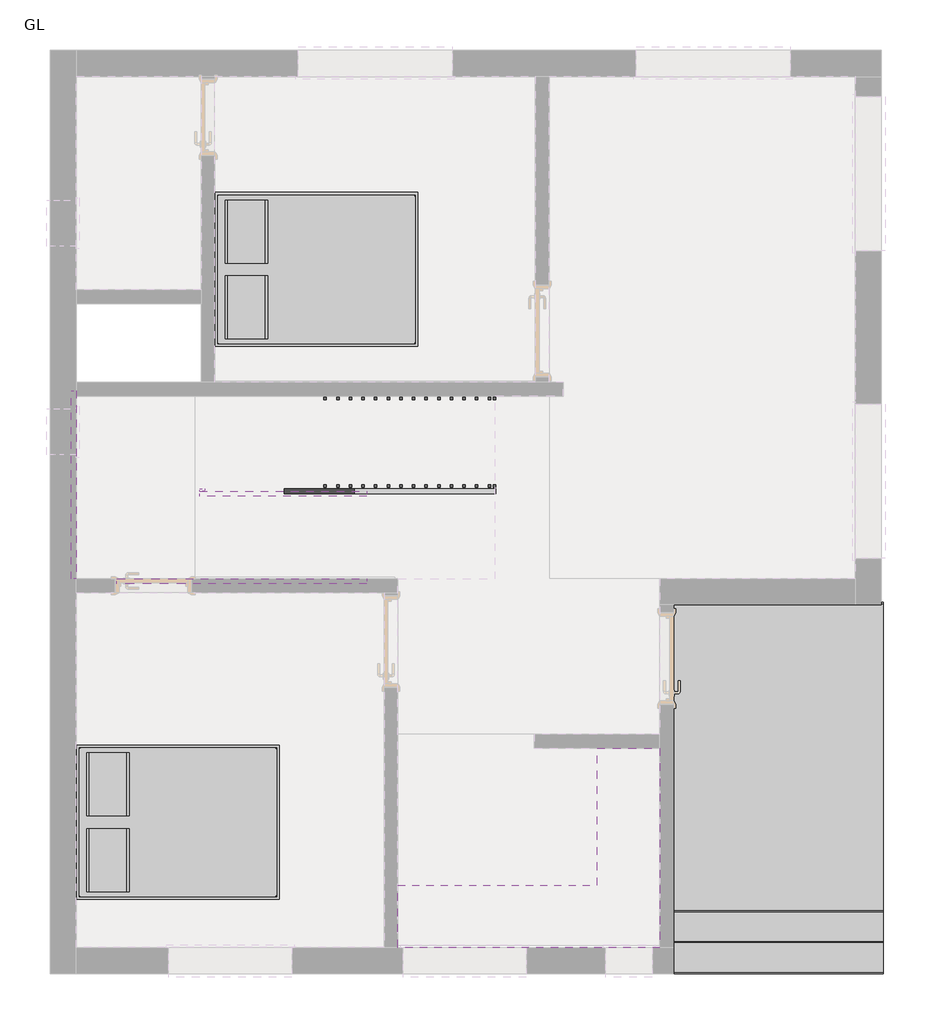
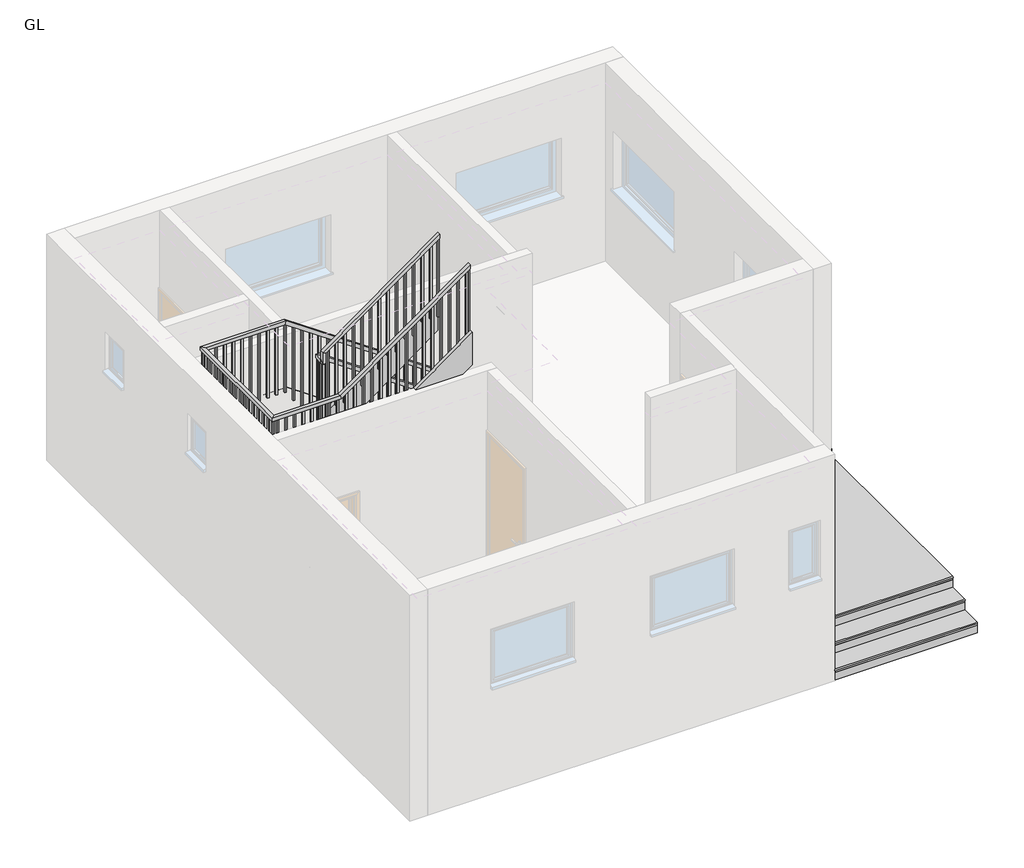
# One storey, part 2 of 2: 6 members, 2 furniture elements, 2 railings, 1 proxy, 1 stair flight.
"""IFC4 building model written with IfcOpenShell, lengths in millimetres."""

from ifc_helpers import new_model, si_unit, frame, origin, place, context, project, spatial, polyline, outline, extrude, faceted_brep, transform, mapped, element, save
from components import generic_models_1_generic_models_1_a00969f3, furniture_bed_1_1525x2007x355mm_queen_b7403446, wood_steps_w_50mm_tread_10mm_nosing_13mm_riser_5aef8f96

model = new_model("IFC4")

# Units and contexts
model_context = context("Model", 3, world=origin())
ifc_project = project(units=[si_unit("LENGTHUNIT", "METRE", prefix="MILLI")], contexts=[model_context])

# Site, building, storey
site = spatial("IfcSite", under=ifc_project)
building = spatial("IfcBuilding", under=site)
storey = spatial("IfcBuildingStorey", under=building, Name="GL", Elevation=0.0)

# Proxy
placement = place(None, origin())
generic_models_1_generic_models_1_shape = generic_models_1_generic_models_1_a00969f3(model_context)
element("IfcBuildingElementProxy", 1, Name="Generic Models 1 : Generic Models 1", ObjectType="Generic Models 1 : Generic Models 1", at=placement, inside=storey, context=model_context, shape_type="MappedRepresentation", body=[
    mapped(generic_models_1_generic_models_1_shape, transform((0.0, 0.0, 0.0), x_axis=(1.0, 0.0, 0.0), y_axis=(0.0, 1.0, 0.0), z_axis=(0.0, 0.0, 1.0))),
])

# Furniture
furniture_bed_1_1525x2007x355mm_queen_shape = furniture_bed_1_1525x2007x355mm_queen_b7403446(model_context)
element("IfcFurniture", 2, ObjectType="Furniture_Bed_1 : 1525x2007x355mm-Queen", at=placement, inside=storey, context=model_context, shape_type="MappedRepresentation", body=[
    mapped(furniture_bed_1_1525x2007x355mm_queen_shape, transform((-8898.6799313, 8340.8671174, 149.9616), x_axis=(0.0, 1.0, 0.0), y_axis=(-1.0, 0.0, 0.0), z_axis=(0.0, 0.0, 1.0))),
])
element("IfcFurniture", 3, ObjectType="Furniture_Bed_1 : 1525x2007x355mm-Queen", at=placement, inside=storey, context=model_context, shape_type="MappedRepresentation", body=[
    mapped(furniture_bed_1_1525x2007x355mm_queen_shape, transform((-10270.2799313, 2866.1131635, 149.9616), x_axis=(0.0, 1.0, 0.0), y_axis=(-1.0, 0.0, 0.0), z_axis=(0.0, 0.0, 1.0))),
])

# Members
element("IfcMember", 4, ObjectType="Stringer-50mm_Width", at=placement, inside=storey, context=model_context, shape_type="SweptSolid", body=[
    extrude(outline(polyline([(0.0, -6888.9904231), (228.9871217, -6888.9904231), (2233.7240638, -9767.6104231), (1746.2809583, -9767.6104231), (0.0, -7260.1097198), (0.0, -6888.9904231)])), frame((0.0, 6457.7656226, 0.0), z_axis=(0.0, 1.0, 0.0), x_axis=(0.0, 0.0, 1.0)), (0.0, 0.0, 1.0), 50.0),
])
element("IfcMember", 5, ObjectType="Stringer-50mm_Width", at=placement, inside=storey, context=model_context, shape_type="SweptSolid", body=[
    extrude(outline(polyline([(-9817.6104231, 6507.7656226), (-9767.6104231, 6507.7656226), (-9767.6104231, 6481.5656226), (-9817.6104231, 6481.5656226), (-9817.6104231, 6507.7656226)])), frame((0.0, 0.0, 1843.7698415), z_axis=(0.0, 0.0, 1.0), x_axis=(1.0, 0.0, 0.0)), (0.0, 0.0, 1.0), 400.0),
])
element("IfcMember", 6, ObjectType="Stringer-50mm_Width", at=placement, inside=storey, context=model_context, shape_type="SweptSolid", body=[
    extrude(outline(polyline([(2441.6210321, -9817.6104231), (1947.0221045, -9817.6104231), (3150.0584681, -8163.4354231), (3644.6573957, -8163.4354231), (2441.6210321, -9817.6104231)])), frame((0.0, 6431.5656226, 0.0), z_axis=(0.0, 1.0, 0.0), x_axis=(0.0, 0.0, 1.0)), (0.0, 0.0, 1.0), 50.0),
])
element("IfcMember", 7, ObjectType="Stringer-50mm_Width", at=placement, inside=storey, context=model_context, shape_type="SweptSolid", body=[
    extrude(outline(polyline([(0.0, -6888.9904231), (228.9871217, -6888.9904231), (2243.7698415, -9782.0352466), (2243.7698415, -10481.9592331), (0.0, -7260.1097198), (0.0, -6888.9904231)])), frame((0.0, 7426.4671174, 0.0), z_axis=(0.0, 1.0, 0.0), x_axis=(0.0, 0.0, 1.0)), (0.0, 0.0, 1.0), 50.0),
])
element("IfcMember", 8, ObjectType="Stringer-50mm_Width", at=placement, inside=storey, context=model_context, shape_type="SweptSolid", body=[
    extrude(outline(polyline([(-11089.3504231, 7476.4671174), (-11039.3504231, 7476.4671174), (-11039.3504231, 5614.7791611), (-11089.3504231, 5614.7791611), (-11089.3504231, 7476.4671174)])), frame((0.0, 0.0, 1843.7698415), z_axis=(0.0, 0.0, 1.0), x_axis=(1.0, 0.0, 0.0)), (0.0, 0.0, 1.0), 400.0),
])
element("IfcMember", 9, ObjectType="Stringer-50mm_Width", at=placement, inside=storey, context=model_context, shape_type="SweptSolid", body=[
    extrude(outline(polyline([(1843.7698415, -9959.5822848), (3150.0584681, -8163.4354231), (3644.6573957, -8163.4354231), (1843.7698415, -10639.6558102), (1843.7698415, -9959.5822848)])), frame((0.0, 5564.7791611, 0.0), z_axis=(0.0, 1.0, 0.0), x_axis=(0.0, 0.0, 1.0)), (0.0, 0.0, 1.0), 50.0),
])

# Railings
element("IfcRailing", 10, ObjectType="1100mm", at=placement, inside=storey, context=model_context, shape_type="SolidModel", body=[
    faceted_brep([(-6888.9904231, 7376.0671174, 1269.3333333), (-6888.9904231, 7376.0671174, 1208.4765973), (-6888.9904231, 7426.0671174, 1208.4765973), (-6888.9904231, 7426.0671174, 1269.3333333), (-9817.6104231, 7376.0671174, 3301.3333333), (-9833.257694, 7376.0671174, 3251.3333333), (-9833.257694, 7426.0671174, 3251.3333333), (-9817.6104231, 7426.0671174, 3301.3333333), (-10988.9504231, 7376.0671174, 3301.3333333), (-10988.9504231, 7376.0671174, 3251.3333333), (-11038.9504231, 7426.0671174, 3251.3333333), (-11038.9504231, 7426.0671174, 3301.3333333), (-10988.9504231, 5665.1791611, 3301.3333333), (-10988.9504231, 5665.1791611, 3251.3333333), (-11038.9504231, 5615.1791611, 3251.3333333), (-11038.9504231, 5615.1791611, 3301.3333333), (-10053.9211374, 5665.1791611, 3301.3333333), (-10037.8562094, 5665.1791611, 3251.3333333), (-10037.8562094, 5615.1791611, 3251.3333333), (-10053.9211374, 5615.1791611, 3301.3333333), (-8163.4354231, 5665.1791611, 4656.0), (-8163.4354231, 5615.1791611, 4656.0), (-8163.4354231, 5615.1791611, 4594.4883433), (-8163.4354231, 5665.1791611, 4594.4883433)], [[[0, 1, 2, 3]], [[1, 0, 4, 5]], [[2, 1, 5, 6]], [[3, 2, 6, 7]], [[0, 3, 7, 4]], [[5, 4, 8, 9]], [[6, 5, 9, 10]], [[7, 6, 10, 11]], [[4, 7, 11, 8]], [[9, 8, 12, 13]], [[10, 9, 13, 14]], [[11, 10, 14, 15]], [[8, 11, 15, 12]], [[13, 12, 16, 17]], [[14, 13, 17, 18]], [[15, 14, 18, 19]], [[12, 15, 19, 16]], [[20, 21, 22, 23]], [[17, 16, 20, 23]], [[18, 17, 23, 22]], [[19, 18, 22, 21]], [[16, 19, 21, 20]]]),
    extrude(outline(polyline([(4558.2907745, -8213.9504231), (3386.6666667, -8213.9504231), (3386.6666667, -8188.9504231), (4576.2050419, -8188.9504231), (4558.2907745, -8213.9504231)])), frame((0.0, 5627.6791611, 0.0), z_axis=(0.0, 1.0, 0.0), x_axis=(0.0, 0.0, 1.0)), (0.0, 0.0, 1.0), 25.0),
    extrude(outline(polyline([(4468.7194373, -8338.9504231), (3386.6666667, -8338.9504231), (3386.6666667, -8313.9504231), (4486.6337048, -8313.9504231), (4468.7194373, -8338.9504231)])), frame((0.0, 5627.6791611, 0.0), z_axis=(0.0, 1.0, 0.0), x_axis=(0.0, 0.0, 1.0)), (0.0, 0.0, 1.0), 25.0),
    extrude(outline(polyline([(4379.1481002, -8463.9504231), (3217.3333333, -8463.9504231), (3217.3333333, -8438.9504231), (4397.0623676, -8438.9504231), (4379.1481002, -8463.9504231)])), frame((0.0, 5627.6791611, 0.0), z_axis=(0.0, 1.0, 0.0), x_axis=(0.0, 0.0, 1.0)), (0.0, 0.0, 1.0), 25.0),
    extrude(outline(polyline([(4289.576763, -8588.9504231), (3217.3333333, -8588.9504231), (3217.3333333, -8563.9504231), (4307.4910304, -8563.9504231), (4289.576763, -8588.9504231)])), frame((0.0, 5627.6791611, 0.0), z_axis=(0.0, 1.0, 0.0), x_axis=(0.0, 0.0, 1.0)), (0.0, 0.0, 1.0), 25.0),
    extrude(outline(polyline([(4200.0054258, -8713.9504231), (3048.0, -8713.9504231), (3048.0, -8688.9504231), (4217.9196933, -8688.9504231), (4200.0054258, -8713.9504231)])), frame((0.0, 5627.6791611, 0.0), z_axis=(0.0, 1.0, 0.0), x_axis=(0.0, 0.0, 1.0)), (0.0, 0.0, 1.0), 25.0),
    extrude(outline(polyline([(4110.4340887, -8838.9504231), (3048.0, -8838.9504231), (3048.0, -8813.9504231), (4128.3483561, -8813.9504231), (4110.4340887, -8838.9504231)])), frame((0.0, 5627.6791611, 0.0), z_axis=(0.0, 1.0, 0.0), x_axis=(0.0, 0.0, 1.0)), (0.0, 0.0, 1.0), 25.0),
    extrude(outline(polyline([(4020.8627515, -8963.9504231), (2878.6666667, -8963.9504231), (2878.6666667, -8938.9504231), (4038.7770189, -8938.9504231), (4020.8627515, -8963.9504231)])), frame((0.0, 5627.6791611, 0.0), z_axis=(0.0, 1.0, 0.0), x_axis=(0.0, 0.0, 1.0)), (0.0, 0.0, 1.0), 25.0),
    extrude(outline(polyline([(3931.2914143, -9088.9504231), (2878.6666667, -9088.9504231), (2878.6666667, -9063.9504231), (3949.2056817, -9063.9504231), (3931.2914143, -9088.9504231)])), frame((0.0, 5627.6791611, 0.0), z_axis=(0.0, 1.0, 0.0), x_axis=(0.0, 0.0, 1.0)), (0.0, 0.0, 1.0), 25.0),
    extrude(outline(polyline([(3841.7200771, -9213.9504231), (2709.3333333, -9213.9504231), (2709.3333333, -9188.9504231), (3859.6343446, -9188.9504231), (3841.7200771, -9213.9504231)])), frame((0.0, 5627.6791611, 0.0), z_axis=(0.0, 1.0, 0.0), x_axis=(0.0, 0.0, 1.0)), (0.0, 0.0, 1.0), 25.0),
    extrude(outline(polyline([(3752.14874, -9338.9504231), (2709.3333333, -9338.9504231), (2709.3333333, -9313.9504231), (3770.0630074, -9313.9504231), (3752.14874, -9338.9504231)])), frame((0.0, 5627.6791611, 0.0), z_axis=(0.0, 1.0, 0.0), x_axis=(0.0, 0.0, 1.0)), (0.0, 0.0, 1.0), 25.0),
    extrude(outline(polyline([(3662.5774028, -9463.9504231), (2540.0, -9463.9504231), (2540.0, -9438.9504231), (3680.4916702, -9438.9504231), (3662.5774028, -9463.9504231)])), frame((0.0, 5627.6791611, 0.0), z_axis=(0.0, 1.0, 0.0), x_axis=(0.0, 0.0, 1.0)), (0.0, 0.0, 1.0), 25.0),
    extrude(outline(polyline([(3573.0060656, -9588.9504231), (2540.0, -9588.9504231), (2540.0, -9563.9504231), (3590.9203331, -9563.9504231), (3573.0060656, -9588.9504231)])), frame((0.0, 5627.6791611, 0.0), z_axis=(0.0, 1.0, 0.0), x_axis=(0.0, 0.0, 1.0)), (0.0, 0.0, 1.0), 25.0),
    extrude(outline(polyline([(3483.4347284, -9713.9504231), (2370.6666667, -9713.9504231), (2370.6666667, -9688.9504231), (3501.3489959, -9688.9504231), (3483.4347284, -9713.9504231)])), frame((0.0, 5627.6791611, 0.0), z_axis=(0.0, 1.0, 0.0), x_axis=(0.0, 0.0, 1.0)), (0.0, 0.0, 1.0), 25.0),
    extrude(outline(polyline([(3393.8633913, -9838.9504231), (2201.3333333, -9838.9504231), (2201.3333333, -9813.9504231), (3411.7776587, -9813.9504231), (3393.8633913, -9838.9504231)])), frame((0.0, 5627.6791611, 0.0), z_axis=(0.0, 1.0, 0.0), x_axis=(0.0, 0.0, 1.0)), (0.0, 0.0, 1.0), 25.0),
    extrude(outline(polyline([(3304.2920541, -9963.9504231), (2201.3333333, -9963.9504231), (2201.3333333, -9938.9504231), (3322.2063215, -9938.9504231), (3304.2920541, -9963.9504231)])), frame((0.0, 5627.6791611, 0.0), z_axis=(0.0, 1.0, 0.0), x_axis=(0.0, 0.0, 1.0)), (0.0, 0.0, 1.0), 25.0),
    extrude(outline(polyline([(-10088.9504231, 5627.6791611), (-10088.9504231, 5652.6791611), (-10063.9504231, 5652.6791611), (-10063.9504231, 5627.6791611), (-10088.9504231, 5627.6791611)])), frame((0.0, 0.0, 2201.3333333), z_axis=(0.0, 0.0, 1.0), x_axis=(1.0, 0.0, 0.0)), (0.0, 0.0, 1.0), 1050.0),
    extrude(outline(polyline([(-10213.9504231, 5627.6791611), (-10213.9504231, 5652.6791611), (-10188.9504231, 5652.6791611), (-10188.9504231, 5627.6791611), (-10213.9504231, 5627.6791611)])), frame((0.0, 0.0, 2201.3333333), z_axis=(0.0, 0.0, 1.0), x_axis=(1.0, 0.0, 0.0)), (0.0, 0.0, 1.0), 1050.0),
    extrude(outline(polyline([(-10338.9504231, 5627.6791611), (-10338.9504231, 5652.6791611), (-10313.9504231, 5652.6791611), (-10313.9504231, 5627.6791611), (-10338.9504231, 5627.6791611)])), frame((0.0, 0.0, 2201.3333333), z_axis=(0.0, 0.0, 1.0), x_axis=(1.0, 0.0, 0.0)), (0.0, 0.0, 1.0), 1050.0),
    extrude(outline(polyline([(-10463.9504231, 5627.6791611), (-10463.9504231, 5652.6791611), (-10438.9504231, 5652.6791611), (-10438.9504231, 5627.6791611), (-10463.9504231, 5627.6791611)])), frame((0.0, 0.0, 2201.3333333), z_axis=(0.0, 0.0, 1.0), x_axis=(1.0, 0.0, 0.0)), (0.0, 0.0, 1.0), 1050.0),
    extrude(outline(polyline([(-10588.9504231, 5627.6791611), (-10588.9504231, 5652.6791611), (-10563.9504231, 5652.6791611), (-10563.9504231, 5627.6791611), (-10588.9504231, 5627.6791611)])), frame((0.0, 0.0, 2201.3333333), z_axis=(0.0, 0.0, 1.0), x_axis=(1.0, 0.0, 0.0)), (0.0, 0.0, 1.0), 1050.0),
    extrude(outline(polyline([(-10713.9504231, 5627.6791611), (-10713.9504231, 5652.6791611), (-10688.9504231, 5652.6791611), (-10688.9504231, 5627.6791611), (-10713.9504231, 5627.6791611)])), frame((0.0, 0.0, 2201.3333333), z_axis=(0.0, 0.0, 1.0), x_axis=(1.0, 0.0, 0.0)), (0.0, 0.0, 1.0), 1050.0),
    extrude(outline(polyline([(-10838.9504231, 5627.6791611), (-10838.9504231, 5652.6791611), (-10813.9504231, 5652.6791611), (-10813.9504231, 5627.6791611), (-10838.9504231, 5627.6791611)])), frame((0.0, 0.0, 2201.3333333), z_axis=(0.0, 0.0, 1.0), x_axis=(1.0, 0.0, 0.0)), (0.0, 0.0, 1.0), 1050.0),
    extrude(outline(polyline([(-10963.9504231, 5627.6791611), (-10963.9504231, 5652.6791611), (-10938.9504231, 5652.6791611), (-10938.9504231, 5627.6791611), (-10963.9504231, 5627.6791611)])), frame((0.0, 0.0, 2201.3333333), z_axis=(0.0, 0.0, 1.0), x_axis=(1.0, 0.0, 0.0)), (0.0, 0.0, 1.0), 1050.0),
    extrude(outline(polyline([(-11026.4504231, 5726.0671174), (-11001.4504231, 5726.0671174), (-11001.4504231, 5701.0671174), (-11026.4504231, 5701.0671174), (-11026.4504231, 5726.0671174)])), frame((0.0, 0.0, 2201.3333333), z_axis=(0.0, 0.0, 1.0), x_axis=(1.0, 0.0, 0.0)), (0.0, 0.0, 1.0), 1050.0),
    extrude(outline(polyline([(-11026.4504231, 5851.0671174), (-11001.4504231, 5851.0671174), (-11001.4504231, 5826.0671174), (-11026.4504231, 5826.0671174), (-11026.4504231, 5851.0671174)])), frame((0.0, 0.0, 2201.3333333), z_axis=(0.0, 0.0, 1.0), x_axis=(1.0, 0.0, 0.0)), (0.0, 0.0, 1.0), 1050.0),
    extrude(outline(polyline([(-11026.4504231, 5976.0671174), (-11001.4504231, 5976.0671174), (-11001.4504231, 5951.0671174), (-11026.4504231, 5951.0671174), (-11026.4504231, 5976.0671174)])), frame((0.0, 0.0, 2201.3333333), z_axis=(0.0, 0.0, 1.0), x_axis=(1.0, 0.0, 0.0)), (0.0, 0.0, 1.0), 1050.0),
    extrude(outline(polyline([(-11026.4504231, 6101.0671174), (-11001.4504231, 6101.0671174), (-11001.4504231, 6076.0671174), (-11026.4504231, 6076.0671174), (-11026.4504231, 6101.0671174)])), frame((0.0, 0.0, 2201.3333333), z_axis=(0.0, 0.0, 1.0), x_axis=(1.0, 0.0, 0.0)), (0.0, 0.0, 1.0), 1050.0),
    extrude(outline(polyline([(-11026.4504231, 6226.0671174), (-11001.4504231, 6226.0671174), (-11001.4504231, 6201.0671174), (-11026.4504231, 6201.0671174), (-11026.4504231, 6226.0671174)])), frame((0.0, 0.0, 2201.3333333), z_axis=(0.0, 0.0, 1.0), x_axis=(1.0, 0.0, 0.0)), (0.0, 0.0, 1.0), 1050.0),
    extrude(outline(polyline([(-11026.4504231, 6351.0671174), (-11001.4504231, 6351.0671174), (-11001.4504231, 6326.0671174), (-11026.4504231, 6326.0671174), (-11026.4504231, 6351.0671174)])), frame((0.0, 0.0, 2201.3333333), z_axis=(0.0, 0.0, 1.0), x_axis=(1.0, 0.0, 0.0)), (0.0, 0.0, 1.0), 1050.0),
    extrude(outline(polyline([(-11026.4504231, 6476.0671174), (-11001.4504231, 6476.0671174), (-11001.4504231, 6451.0671174), (-11026.4504231, 6451.0671174), (-11026.4504231, 6476.0671174)])), frame((0.0, 0.0, 2201.3333333), z_axis=(0.0, 0.0, 1.0), x_axis=(1.0, 0.0, 0.0)), (0.0, 0.0, 1.0), 1050.0),
    extrude(outline(polyline([(-11026.4504231, 6601.0671174), (-11001.4504231, 6601.0671174), (-11001.4504231, 6576.0671174), (-11026.4504231, 6576.0671174), (-11026.4504231, 6601.0671174)])), frame((0.0, 0.0, 2201.3333333), z_axis=(0.0, 0.0, 1.0), x_axis=(1.0, 0.0, 0.0)), (0.0, 0.0, 1.0), 1050.0),
    extrude(outline(polyline([(-11026.4504231, 6726.0671174), (-11001.4504231, 6726.0671174), (-11001.4504231, 6701.0671174), (-11026.4504231, 6701.0671174), (-11026.4504231, 6726.0671174)])), frame((0.0, 0.0, 2201.3333333), z_axis=(0.0, 0.0, 1.0), x_axis=(1.0, 0.0, 0.0)), (0.0, 0.0, 1.0), 1050.0),
    extrude(outline(polyline([(-11026.4504231, 6851.0671174), (-11001.4504231, 6851.0671174), (-11001.4504231, 6826.0671174), (-11026.4504231, 6826.0671174), (-11026.4504231, 6851.0671174)])), frame((0.0, 0.0, 2201.3333333), z_axis=(0.0, 0.0, 1.0), x_axis=(1.0, 0.0, 0.0)), (0.0, 0.0, 1.0), 1050.0),
    extrude(outline(polyline([(-11026.4504231, 6976.0671174), (-11001.4504231, 6976.0671174), (-11001.4504231, 6951.0671174), (-11026.4504231, 6951.0671174), (-11026.4504231, 6976.0671174)])), frame((0.0, 0.0, 2201.3333333), z_axis=(0.0, 0.0, 1.0), x_axis=(1.0, 0.0, 0.0)), (0.0, 0.0, 1.0), 1050.0),
    extrude(outline(polyline([(-11026.4504231, 7101.0671174), (-11001.4504231, 7101.0671174), (-11001.4504231, 7076.0671174), (-11026.4504231, 7076.0671174), (-11026.4504231, 7101.0671174)])), frame((0.0, 0.0, 2201.3333333), z_axis=(0.0, 0.0, 1.0), x_axis=(1.0, 0.0, 0.0)), (0.0, 0.0, 1.0), 1050.0),
    extrude(outline(polyline([(-11026.4504231, 7226.0671174), (-11001.4504231, 7226.0671174), (-11001.4504231, 7201.0671174), (-11026.4504231, 7201.0671174), (-11026.4504231, 7226.0671174)])), frame((0.0, 0.0, 2201.3333333), z_axis=(0.0, 0.0, 1.0), x_axis=(1.0, 0.0, 0.0)), (0.0, 0.0, 1.0), 1050.0),
    extrude(outline(polyline([(-11026.4504231, 7351.0671174), (-11001.4504231, 7351.0671174), (-11001.4504231, 7326.0671174), (-11026.4504231, 7326.0671174), (-11026.4504231, 7351.0671174)])), frame((0.0, 0.0, 2201.3333333), z_axis=(0.0, 0.0, 1.0), x_axis=(1.0, 0.0, 0.0)), (0.0, 0.0, 1.0), 1050.0),
    extrude(outline(polyline([(-10938.9904231, 7413.5671174), (-10938.9904231, 7388.5671174), (-10963.9904231, 7388.5671174), (-10963.9904231, 7413.5671174), (-10938.9904231, 7413.5671174)])), frame((0.0, 0.0, 2201.3333333), z_axis=(0.0, 0.0, 1.0), x_axis=(1.0, 0.0, 0.0)), (0.0, 0.0, 1.0), 1050.0),
    extrude(outline(polyline([(-10813.9904231, 7413.5671174), (-10813.9904231, 7388.5671174), (-10838.9904231, 7388.5671174), (-10838.9904231, 7413.5671174), (-10813.9904231, 7413.5671174)])), frame((0.0, 0.0, 2201.3333333), z_axis=(0.0, 0.0, 1.0), x_axis=(1.0, 0.0, 0.0)), (0.0, 0.0, 1.0), 1050.0),
    extrude(outline(polyline([(-10688.9904231, 7413.5671174), (-10688.9904231, 7388.5671174), (-10713.9904231, 7388.5671174), (-10713.9904231, 7413.5671174), (-10688.9904231, 7413.5671174)])), frame((0.0, 0.0, 2201.3333333), z_axis=(0.0, 0.0, 1.0), x_axis=(1.0, 0.0, 0.0)), (0.0, 0.0, 1.0), 1050.0),
    extrude(outline(polyline([(-10563.9904231, 7413.5671174), (-10563.9904231, 7388.5671174), (-10588.9904231, 7388.5671174), (-10588.9904231, 7413.5671174), (-10563.9904231, 7413.5671174)])), frame((0.0, 0.0, 2201.3333333), z_axis=(0.0, 0.0, 1.0), x_axis=(1.0, 0.0, 0.0)), (0.0, 0.0, 1.0), 1050.0),
    extrude(outline(polyline([(-10438.9904231, 7413.5671174), (-10438.9904231, 7388.5671174), (-10463.9904231, 7388.5671174), (-10463.9904231, 7413.5671174), (-10438.9904231, 7413.5671174)])), frame((0.0, 0.0, 2201.3333333), z_axis=(0.0, 0.0, 1.0), x_axis=(1.0, 0.0, 0.0)), (0.0, 0.0, 1.0), 1050.0),
    extrude(outline(polyline([(-10313.9904231, 7413.5671174), (-10313.9904231, 7388.5671174), (-10338.9904231, 7388.5671174), (-10338.9904231, 7413.5671174), (-10313.9904231, 7413.5671174)])), frame((0.0, 0.0, 2201.3333333), z_axis=(0.0, 0.0, 1.0), x_axis=(1.0, 0.0, 0.0)), (0.0, 0.0, 1.0), 1050.0),
    extrude(outline(polyline([(-10188.9904231, 7413.5671174), (-10188.9904231, 7388.5671174), (-10213.9904231, 7388.5671174), (-10213.9904231, 7413.5671174), (-10188.9904231, 7413.5671174)])), frame((0.0, 0.0, 2201.3333333), z_axis=(0.0, 0.0, 1.0), x_axis=(1.0, 0.0, 0.0)), (0.0, 0.0, 1.0), 1050.0),
    extrude(outline(polyline([(-10063.9904231, 7413.5671174), (-10063.9904231, 7388.5671174), (-10088.9904231, 7388.5671174), (-10088.9904231, 7413.5671174), (-10063.9904231, 7413.5671174)])), frame((0.0, 0.0, 2201.3333333), z_axis=(0.0, 0.0, 1.0), x_axis=(1.0, 0.0, 0.0)), (0.0, 0.0, 1.0), 1050.0),
    extrude(outline(polyline([(-9938.9904231, 7413.5671174), (-9938.9904231, 7388.5671174), (-9963.9904231, 7388.5671174), (-9963.9904231, 7413.5671174), (-9938.9904231, 7413.5671174)])), frame((0.0, 0.0, 2201.3333333), z_axis=(0.0, 0.0, 1.0), x_axis=(1.0, 0.0, 0.0)), (0.0, 0.0, 1.0), 1050.0),
    extrude(outline(polyline([(-9813.9904231, 7413.5671174), (-9813.9904231, 7388.5671174), (-9838.9904231, 7388.5671174), (-9838.9904231, 7413.5671174), (-9813.9904231, 7413.5671174)])), frame((0.0, 0.0, 2201.3333333), z_axis=(0.0, 0.0, 1.0), x_axis=(1.0, 0.0, 0.0)), (0.0, 0.0, 1.0), 1050.0),
    extrude(outline(polyline([(2032.0, -9688.9904231), (3151.2346198, -9688.9904231), (3168.5806736, -9713.9904231), (2032.0, -9713.9904231), (2032.0, -9688.9904231)])), frame((0.0, 7388.5671174, 0.0), z_axis=(0.0, 1.0, 0.0), x_axis=(0.0, 0.0, 1.0)), (0.0, 0.0, 1.0), 25.0),
    extrude(outline(polyline([(1862.6666667, -9563.9904231), (3064.5043509, -9563.9904231), (3081.8504047, -9588.9904231), (1862.6666667, -9588.9904231), (1862.6666667, -9563.9904231)])), frame((0.0, 7388.5671174, 0.0), z_axis=(0.0, 1.0, 0.0), x_axis=(0.0, 0.0, 1.0)), (0.0, 0.0, 1.0), 25.0),
    extrude(outline(polyline([(1862.6666667, -9438.9904231), (2977.7740821, -9438.9904231), (2995.1201359, -9463.9904231), (1862.6666667, -9463.9904231), (1862.6666667, -9438.9904231)])), frame((0.0, 7388.5671174, 0.0), z_axis=(0.0, 1.0, 0.0), x_axis=(0.0, 0.0, 1.0)), (0.0, 0.0, 1.0), 25.0),
    extrude(outline(polyline([(1693.3333333, -9313.9904231), (2891.0438132, -9313.9904231), (2908.389867, -9338.9904231), (1693.3333333, -9338.9904231), (1693.3333333, -9313.9904231)])), frame((0.0, 7388.5671174, 0.0), z_axis=(0.0, 1.0, 0.0), x_axis=(0.0, 0.0, 1.0)), (0.0, 0.0, 1.0), 25.0),
    extrude(outline(polyline([(1693.3333333, -9188.9904231), (2804.3135444, -9188.9904231), (2821.6595981, -9213.9904231), (1693.3333333, -9213.9904231), (1693.3333333, -9188.9904231)])), frame((0.0, 7388.5671174, 0.0), z_axis=(0.0, 1.0, 0.0), x_axis=(0.0, 0.0, 1.0)), (0.0, 0.0, 1.0), 25.0),
    extrude(outline(polyline([(1524.0, -9063.9904231), (2717.5832755, -9063.9904231), (2734.9293293, -9088.9904231), (1524.0, -9088.9904231), (1524.0, -9063.9904231)])), frame((0.0, 7388.5671174, 0.0), z_axis=(0.0, 1.0, 0.0), x_axis=(0.0, 0.0, 1.0)), (0.0, 0.0, 1.0), 25.0),
    extrude(outline(polyline([(1524.0, -8938.9904231), (2630.8530066, -8938.9904231), (2648.1990604, -8963.9904231), (1524.0, -8963.9904231), (1524.0, -8938.9904231)])), frame((0.0, 7388.5671174, 0.0), z_axis=(0.0, 1.0, 0.0), x_axis=(0.0, 0.0, 1.0)), (0.0, 0.0, 1.0), 25.0),
    extrude(outline(polyline([(1354.6666667, -8813.9904231), (2544.1227378, -8813.9904231), (2561.4687915, -8838.9904231), (1354.6666667, -8838.9904231), (1354.6666667, -8813.9904231)])), frame((0.0, 7388.5671174, 0.0), z_axis=(0.0, 1.0, 0.0), x_axis=(0.0, 0.0, 1.0)), (0.0, 0.0, 1.0), 25.0),
    extrude(outline(polyline([(1354.6666667, -8688.9904231), (2457.3924689, -8688.9904231), (2474.7385227, -8713.9904231), (1354.6666667, -8713.9904231), (1354.6666667, -8688.9904231)])), frame((0.0, 7388.5671174, 0.0), z_axis=(0.0, 1.0, 0.0), x_axis=(0.0, 0.0, 1.0)), (0.0, 0.0, 1.0), 25.0),
    extrude(outline(polyline([(1185.3333333, -8563.9904231), (2370.6622, -8563.9904231), (2388.0082538, -8588.9904231), (1185.3333333, -8588.9904231), (1185.3333333, -8563.9904231)])), frame((0.0, 7388.5671174, 0.0), z_axis=(0.0, 1.0, 0.0), x_axis=(0.0, 0.0, 1.0)), (0.0, 0.0, 1.0), 25.0),
    extrude(outline(polyline([(1185.3333333, -8438.9904231), (2283.9319312, -8438.9904231), (2301.2779849, -8463.9904231), (1185.3333333, -8463.9904231), (1185.3333333, -8438.9904231)])), frame((0.0, 7388.5671174, 0.0), z_axis=(0.0, 1.0, 0.0), x_axis=(0.0, 0.0, 1.0)), (0.0, 0.0, 1.0), 25.0),
    extrude(outline(polyline([(1016.0, -8313.9904231), (2197.2016623, -8313.9904231), (2214.5477161, -8338.9904231), (1016.0, -8338.9904231), (1016.0, -8313.9904231)])), frame((0.0, 7388.5671174, 0.0), z_axis=(0.0, 1.0, 0.0), x_axis=(0.0, 0.0, 1.0)), (0.0, 0.0, 1.0), 25.0),
    extrude(outline(polyline([(1016.0, -8188.9904231), (2110.4713934, -8188.9904231), (2127.8174472, -8213.9904231), (1016.0, -8213.9904231), (1016.0, -8188.9904231)])), frame((0.0, 7388.5671174, 0.0), z_axis=(0.0, 1.0, 0.0), x_axis=(0.0, 0.0, 1.0)), (0.0, 0.0, 1.0), 25.0),
    extrude(outline(polyline([(846.6666667, -8063.9904231), (2023.7411246, -8063.9904231), (2041.0871783, -8088.9904231), (846.6666667, -8088.9904231), (846.6666667, -8063.9904231)])), frame((0.0, 7388.5671174, 0.0), z_axis=(0.0, 1.0, 0.0), x_axis=(0.0, 0.0, 1.0)), (0.0, 0.0, 1.0), 25.0),
    extrude(outline(polyline([(846.6666667, -7938.9904231), (1937.0108557, -7938.9904231), (1954.3569095, -7963.9904231), (846.6666667, -7963.9904231), (846.6666667, -7938.9904231)])), frame((0.0, 7388.5671174, 0.0), z_axis=(0.0, 1.0, 0.0), x_axis=(0.0, 0.0, 1.0)), (0.0, 0.0, 1.0), 25.0),
    extrude(outline(polyline([(677.3333333, -7813.9904231), (1850.2805868, -7813.9904231), (1867.6266406, -7838.9904231), (677.3333333, -7838.9904231), (677.3333333, -7813.9904231)])), frame((0.0, 7388.5671174, 0.0), z_axis=(0.0, 1.0, 0.0), x_axis=(0.0, 0.0, 1.0)), (0.0, 0.0, 1.0), 25.0),
    extrude(outline(polyline([(677.3333333, -7688.9904231), (1763.550318, -7688.9904231), (1780.8963718, -7713.9904231), (677.3333333, -7713.9904231), (677.3333333, -7688.9904231)])), frame((0.0, 7388.5671174, 0.0), z_axis=(0.0, 1.0, 0.0), x_axis=(0.0, 0.0, 1.0)), (0.0, 0.0, 1.0), 25.0),
    extrude(outline(polyline([(508.0, -7563.9904231), (1676.8200491, -7563.9904231), (1694.1661029, -7588.9904231), (508.0, -7588.9904231), (508.0, -7563.9904231)])), frame((0.0, 7388.5671174, 0.0), z_axis=(0.0, 1.0, 0.0), x_axis=(0.0, 0.0, 1.0)), (0.0, 0.0, 1.0), 25.0),
    extrude(outline(polyline([(508.0, -7438.9904231), (1590.0897803, -7438.9904231), (1607.435834, -7463.9904231), (508.0, -7463.9904231), (508.0, -7438.9904231)])), frame((0.0, 7388.5671174, 0.0), z_axis=(0.0, 1.0, 0.0), x_axis=(0.0, 0.0, 1.0)), (0.0, 0.0, 1.0), 25.0),
    extrude(outline(polyline([(338.6666667, -7313.9904231), (1503.3595114, -7313.9904231), (1520.7055652, -7338.9904231), (338.6666667, -7338.9904231), (338.6666667, -7313.9904231)])), frame((0.0, 7388.5671174, 0.0), z_axis=(0.0, 1.0, 0.0), x_axis=(0.0, 0.0, 1.0)), (0.0, 0.0, 1.0), 25.0),
    extrude(outline(polyline([(338.6666667, -7188.9904231), (1416.6292425, -7188.9904231), (1433.9752963, -7213.9904231), (338.6666667, -7213.9904231), (338.6666667, -7188.9904231)])), frame((0.0, 7388.5671174, 0.0), z_axis=(0.0, 1.0, 0.0), x_axis=(0.0, 0.0, 1.0)), (0.0, 0.0, 1.0), 25.0),
    extrude(outline(polyline([(169.3333333, -7063.9904231), (1329.8989737, -7063.9904231), (1347.2450274, -7088.9904231), (169.3333333, -7088.9904231), (169.3333333, -7063.9904231)])), frame((0.0, 7388.5671174, 0.0), z_axis=(0.0, 1.0, 0.0), x_axis=(0.0, 0.0, 1.0)), (0.0, 0.0, 1.0), 25.0),
    extrude(outline(polyline([(169.3333333, -6938.9904231), (1243.1687048, -6938.9904231), (1260.5147586, -6963.9904231), (169.3333333, -6963.9904231), (169.3333333, -6938.9904231)])), frame((0.0, 7388.5671174, 0.0), z_axis=(0.0, 1.0, 0.0), x_axis=(0.0, 0.0, 1.0)), (0.0, 0.0, 1.0), 25.0),
    extrude(outline(polyline([(-11026.4504231, 5652.6791611), (-11001.4504231, 5652.6791611), (-11001.4504231, 5627.6791611), (-11026.4504231, 5627.6791611), (-11026.4504231, 5652.6791611)])), frame((0.0, 0.0, 2201.3333333), z_axis=(0.0, 0.0, 1.0), x_axis=(1.0, 0.0, 0.0)), (0.0, 0.0, 1.0), 1050.0),
    extrude(outline(polyline([(-11001.4504231, 7413.5671174), (-11001.4504231, 7388.5671174), (-11026.4504231, 7388.5671174), (-11026.4504231, 7413.5671174), (-11001.4504231, 7413.5671174)])), frame((0.0, 0.0, 2201.3333333), z_axis=(0.0, 0.0, 1.0), x_axis=(1.0, 0.0, 0.0)), (0.0, 0.0, 1.0), 1050.0),
    extrude(outline(polyline([(4576.5740759, -8188.4354231), (3386.6666667, -8188.4354231), (3386.6666667, -8163.4354231), (4594.4883433, -8163.4354231), (4576.5740759, -8188.4354231)])), frame((0.0, 5627.6791611, 0.0), z_axis=(0.0, 1.0, 0.0), x_axis=(0.0, 0.0, 1.0)), (0.0, 0.0, 1.0), 25.0),
    extrude(outline(polyline([(169.3333333, -6888.9904231), (1208.4765973, -6888.9904231), (1225.822651, -6913.9904231), (169.3333333, -6913.9904231), (169.3333333, -6888.9904231)])), frame((0.0, 7388.5671174, 0.0), z_axis=(0.0, 1.0, 0.0), x_axis=(0.0, 0.0, 1.0)), (0.0, 0.0, 1.0), 25.0),
])
element("IfcRailing", 11, ObjectType="1100mm", at=placement, inside=storey, context=model_context, shape_type="SolidModel", body=[
    faceted_brep([(-6888.9904231, 6508.1656226, 1269.3333333), (-6888.9904231, 6508.1656226, 1208.4765973), (-6888.9904231, 6558.1656226, 1208.4765973), (-6888.9904231, 6558.1656226, 1269.3333333), (-9743.0104231, 6508.1656226, 3249.5727089), (-9793.0104231, 6508.1656226, 3223.4080803), (-9793.0104231, 6558.1656226, 3223.4080803), (-9743.0104231, 6558.1656226, 3249.5727089), (-9743.0104231, 6508.1656226, 3301.3333333), (-9793.0104231, 6508.1656226, 3251.3333333), (-9793.0104231, 6558.1656226, 3251.3333333), (-9743.0104231, 6558.1656226, 3301.3333333), (-9818.0104231, 6508.1656226, 3301.3333333), (-9818.0104231, 6508.1656226, 3251.3333333), (-9868.0104231, 6558.1656226, 3251.3333333), (-9868.0104231, 6558.1656226, 3301.3333333), (-9818.0104231, 6433.1656226, 3301.3333333), (-9818.0104231, 6433.1656226, 3251.3333333), (-9868.0104231, 6433.1656226, 3251.3333333), (-9868.0104231, 6433.1656226, 3301.3333333), (-9818.0104231, 6431.1656226, 3301.3333333), (-9868.0104231, 6431.1656226, 3301.3333333), (-9868.0104231, 6381.1656226, 3251.3333333), (-9818.0104231, 6381.1656226, 3251.3333333)], [[[0, 1, 2, 3]], [[1, 0, 4, 5]], [[2, 1, 5, 6]], [[3, 2, 6, 7]], [[0, 3, 7, 4]], [[5, 4, 8, 9]], [[6, 5, 9, 10]], [[7, 6, 10, 11]], [[4, 7, 11, 8]], [[9, 8, 12, 13]], [[10, 9, 13, 14]], [[11, 10, 14, 15]], [[8, 11, 15, 12]], [[13, 12, 16, 17]], [[14, 13, 17, 18]], [[15, 14, 18, 19]], [[12, 15, 19, 16]], [[20, 21, 22, 23]], [[17, 16, 20, 23]], [[18, 17, 23, 22]], [[19, 18, 22, 21]], [[16, 19, 21, 20]]]),
    faceted_brep([(-9818.0104231, 6431.1656226, 3301.3333333), (-9818.0104231, 6381.1656226, 3251.3333333), (-9868.0104231, 6381.1656226, 3251.3333333), (-9868.0104231, 6431.1656226, 3301.3333333), (-9818.0104231, 6431.1656226, 3408.8683817), (-9868.0104231, 6431.1656226, 3434.5515035), (-9868.0104231, 6381.1656226, 3434.5515035), (-9818.0104231, 6381.1656226, 3408.8683817)], [[[0, 1, 2, 3]], [[4, 5, 6, 7]], [[1, 0, 4, 7]], [[2, 1, 7, 6]], [[3, 2, 6, 5]], [[0, 3, 5, 4]]]),
    faceted_brep([(-9868.0104231, 6431.1656226, 3434.5515035), (-9818.0104231, 6431.1656226, 3408.8683817), (-9818.0104231, 6381.1656226, 3408.8683817), (-9868.0104231, 6381.1656226, 3434.5515035), (-8163.4354231, 6431.1656226, 4656.0), (-8163.4354231, 6381.1656226, 4656.0), (-8163.4354231, 6381.1656226, 4594.4883433), (-8163.4354231, 6431.1656226, 4594.4883433)], [[[0, 1, 2, 3]], [[4, 5, 6, 7]], [[1, 0, 4, 7]], [[2, 1, 7, 6]], [[3, 2, 6, 5]], [[0, 3, 5, 4]]]),
    extrude(outline(polyline([(3386.6666667, -8293.0104231), (3386.6666667, -8268.0104231), (4519.5529626, -8268.0104231), (4501.6386952, -8293.0104231), (3386.6666667, -8293.0104231)])), frame((0.0, 6393.6656226, 0.0), z_axis=(0.0, 1.0, 0.0), x_axis=(0.0, 0.0, 1.0)), (0.0, 0.0, 1.0), 25.0),
    extrude(outline(polyline([(3386.6666667, -8418.0104231), (3386.6666667, -8393.0104231), (4429.9816254, -8393.0104231), (4412.067358, -8418.0104231), (3386.6666667, -8418.0104231)])), frame((0.0, 6393.6656226, 0.0), z_axis=(0.0, 1.0, 0.0), x_axis=(0.0, 0.0, 1.0)), (0.0, 0.0, 1.0), 25.0),
    extrude(outline(polyline([(3217.3333333, -8543.0104231), (3217.3333333, -8518.0104231), (4340.4102883, -8518.0104231), (4322.4960208, -8543.0104231), (3217.3333333, -8543.0104231)])), frame((0.0, 6393.6656226, 0.0), z_axis=(0.0, 1.0, 0.0), x_axis=(0.0, 0.0, 1.0)), (0.0, 0.0, 1.0), 25.0),
    extrude(outline(polyline([(3217.3333333, -8668.0104231), (3217.3333333, -8643.0104231), (4250.8389511, -8643.0104231), (4232.9246837, -8668.0104231), (3217.3333333, -8668.0104231)])), frame((0.0, 6393.6656226, 0.0), z_axis=(0.0, 1.0, 0.0), x_axis=(0.0, 0.0, 1.0)), (0.0, 0.0, 1.0), 25.0),
    extrude(outline(polyline([(3048.0, -8793.0104231), (3048.0, -8768.0104231), (4161.2676139, -8768.0104231), (4143.3533465, -8793.0104231), (3048.0, -8793.0104231)])), frame((0.0, 6393.6656226, 0.0), z_axis=(0.0, 1.0, 0.0), x_axis=(0.0, 0.0, 1.0)), (0.0, 0.0, 1.0), 25.0),
    extrude(outline(polyline([(3048.0, -8918.0104231), (3048.0, -8893.0104231), (4071.6962768, -8893.0104231), (4053.7820093, -8918.0104231), (3048.0, -8918.0104231)])), frame((0.0, 6393.6656226, 0.0), z_axis=(0.0, 1.0, 0.0), x_axis=(0.0, 0.0, 1.0)), (0.0, 0.0, 1.0), 25.0),
    extrude(outline(polyline([(2878.6666667, -9043.0104231), (2878.6666667, -9018.0104231), (3982.1249396, -9018.0104231), (3964.2106721, -9043.0104231), (2878.6666667, -9043.0104231)])), frame((0.0, 6393.6656226, 0.0), z_axis=(0.0, 1.0, 0.0), x_axis=(0.0, 0.0, 1.0)), (0.0, 0.0, 1.0), 25.0),
    extrude(outline(polyline([(2878.6666667, -9168.0104231), (2878.6666667, -9143.0104231), (3892.5536024, -9143.0104231), (3874.639335, -9168.0104231), (2878.6666667, -9168.0104231)])), frame((0.0, 6393.6656226, 0.0), z_axis=(0.0, 1.0, 0.0), x_axis=(0.0, 0.0, 1.0)), (0.0, 0.0, 1.0), 25.0),
    extrude(outline(polyline([(2709.3333333, -9293.0104231), (2709.3333333, -9268.0104231), (3802.9822652, -9268.0104231), (3785.0679978, -9293.0104231), (2709.3333333, -9293.0104231)])), frame((0.0, 6393.6656226, 0.0), z_axis=(0.0, 1.0, 0.0), x_axis=(0.0, 0.0, 1.0)), (0.0, 0.0, 1.0), 25.0),
    extrude(outline(polyline([(2709.3333333, -9418.0104231), (2709.3333333, -9393.0104231), (3713.4109281, -9393.0104231), (3695.4966606, -9418.0104231), (2709.3333333, -9418.0104231)])), frame((0.0, 6393.6656226, 0.0), z_axis=(0.0, 1.0, 0.0), x_axis=(0.0, 0.0, 1.0)), (0.0, 0.0, 1.0), 25.0),
    extrude(outline(polyline([(2540.0, -9543.0104231), (2540.0, -9518.0104231), (3623.8395909, -9518.0104231), (3605.9253235, -9543.0104231), (2540.0, -9543.0104231)])), frame((0.0, 6393.6656226, 0.0), z_axis=(0.0, 1.0, 0.0), x_axis=(0.0, 0.0, 1.0)), (0.0, 0.0, 1.0), 25.0),
    extrude(outline(polyline([(2540.0, -9668.0104231), (2540.0, -9643.0104231), (3534.2682537, -9643.0104231), (3516.3539863, -9668.0104231), (2540.0, -9668.0104231)])), frame((0.0, 6393.6656226, 0.0), z_axis=(0.0, 1.0, 0.0), x_axis=(0.0, 0.0, 1.0)), (0.0, 0.0, 1.0), 25.0),
    extrude(outline(polyline([(2370.6666667, -9793.0104231), (2370.6666667, -9768.0104231), (3444.6969165, -9768.0104231), (3426.7826491, -9793.0104231), (2370.6666667, -9793.0104231)])), frame((0.0, 6393.6656226, 0.0), z_axis=(0.0, 1.0, 0.0), x_axis=(0.0, 0.0, 1.0)), (0.0, 0.0, 1.0), 25.0),
    extrude(outline(polyline([(-9830.5104231, 6483.1656226), (-9830.5104231, 6458.1656226), (-9855.5104231, 6458.1656226), (-9855.5104231, 6483.1656226), (-9830.5104231, 6483.1656226)])), frame((0.0, 0.0, 2201.3333333), z_axis=(0.0, 0.0, 1.0), x_axis=(1.0, 0.0, 0.0)), (0.0, 0.0, 1.0), 1050.0),
    extrude(outline(polyline([(-9813.9904231, 6520.6656226), (-9838.9904231, 6520.6656226), (-9838.9904231, 6545.6656226), (-9813.9904231, 6545.6656226), (-9813.9904231, 6520.6656226)])), frame((0.0, 0.0, 2201.3333333), z_axis=(0.0, 0.0, 1.0), x_axis=(1.0, 0.0, 0.0)), (0.0, 0.0, 1.0), 1050.0),
    extrude(outline(polyline([(3151.2346198, -9688.9904231), (3168.5806736, -9713.9904231), (2032.0, -9713.9904231), (2032.0, -9688.9904231), (3151.2346198, -9688.9904231)])), frame((0.0, 6520.6656226, 0.0), z_axis=(0.0, 1.0, 0.0), x_axis=(0.0, 0.0, 1.0)), (0.0, 0.0, 1.0), 25.0),
    extrude(outline(polyline([(3064.5043509, -9563.9904231), (3081.8504047, -9588.9904231), (1862.6666667, -9588.9904231), (1862.6666667, -9563.9904231), (3064.5043509, -9563.9904231)])), frame((0.0, 6520.6656226, 0.0), z_axis=(0.0, 1.0, 0.0), x_axis=(0.0, 0.0, 1.0)), (0.0, 0.0, 1.0), 25.0),
    extrude(outline(polyline([(2977.7740821, -9438.9904231), (2995.1201359, -9463.9904231), (1862.6666667, -9463.9904231), (1862.6666667, -9438.9904231), (2977.7740821, -9438.9904231)])), frame((0.0, 6520.6656226, 0.0), z_axis=(0.0, 1.0, 0.0), x_axis=(0.0, 0.0, 1.0)), (0.0, 0.0, 1.0), 25.0),
    extrude(outline(polyline([(2891.0438132, -9313.9904231), (2908.389867, -9338.9904231), (1693.3333333, -9338.9904231), (1693.3333333, -9313.9904231), (2891.0438132, -9313.9904231)])), frame((0.0, 6520.6656226, 0.0), z_axis=(0.0, 1.0, 0.0), x_axis=(0.0, 0.0, 1.0)), (0.0, 0.0, 1.0), 25.0),
    extrude(outline(polyline([(2804.3135444, -9188.9904231), (2821.6595981, -9213.9904231), (1693.3333333, -9213.9904231), (1693.3333333, -9188.9904231), (2804.3135444, -9188.9904231)])), frame((0.0, 6520.6656226, 0.0), z_axis=(0.0, 1.0, 0.0), x_axis=(0.0, 0.0, 1.0)), (0.0, 0.0, 1.0), 25.0),
    extrude(outline(polyline([(2717.5832755, -9063.9904231), (2734.9293293, -9088.9904231), (1524.0, -9088.9904231), (1524.0, -9063.9904231), (2717.5832755, -9063.9904231)])), frame((0.0, 6520.6656226, 0.0), z_axis=(0.0, 1.0, 0.0), x_axis=(0.0, 0.0, 1.0)), (0.0, 0.0, 1.0), 25.0),
    extrude(outline(polyline([(2630.8530066, -8938.9904231), (2648.1990604, -8963.9904231), (1524.0, -8963.9904231), (1524.0, -8938.9904231), (2630.8530066, -8938.9904231)])), frame((0.0, 6520.6656226, 0.0), z_axis=(0.0, 1.0, 0.0), x_axis=(0.0, 0.0, 1.0)), (0.0, 0.0, 1.0), 25.0),
    extrude(outline(polyline([(2544.1227378, -8813.9904231), (2561.4687915, -8838.9904231), (1354.6666667, -8838.9904231), (1354.6666667, -8813.9904231), (2544.1227378, -8813.9904231)])), frame((0.0, 6520.6656226, 0.0), z_axis=(0.0, 1.0, 0.0), x_axis=(0.0, 0.0, 1.0)), (0.0, 0.0, 1.0), 25.0),
    extrude(outline(polyline([(2457.3924689, -8688.9904231), (2474.7385227, -8713.9904231), (1354.6666667, -8713.9904231), (1354.6666667, -8688.9904231), (2457.3924689, -8688.9904231)])), frame((0.0, 6520.6656226, 0.0), z_axis=(0.0, 1.0, 0.0), x_axis=(0.0, 0.0, 1.0)), (0.0, 0.0, 1.0), 25.0),
    extrude(outline(polyline([(2370.6622, -8563.9904231), (2388.0082538, -8588.9904231), (1185.3333333, -8588.9904231), (1185.3333333, -8563.9904231), (2370.6622, -8563.9904231)])), frame((0.0, 6520.6656226, 0.0), z_axis=(0.0, 1.0, 0.0), x_axis=(0.0, 0.0, 1.0)), (0.0, 0.0, 1.0), 25.0),
    extrude(outline(polyline([(2283.9319312, -8438.9904231), (2301.2779849, -8463.9904231), (1185.3333333, -8463.9904231), (1185.3333333, -8438.9904231), (2283.9319312, -8438.9904231)])), frame((0.0, 6520.6656226, 0.0), z_axis=(0.0, 1.0, 0.0), x_axis=(0.0, 0.0, 1.0)), (0.0, 0.0, 1.0), 25.0),
    extrude(outline(polyline([(2197.2016623, -8313.9904231), (2214.5477161, -8338.9904231), (1016.0, -8338.9904231), (1016.0, -8313.9904231), (2197.2016623, -8313.9904231)])), frame((0.0, 6520.6656226, 0.0), z_axis=(0.0, 1.0, 0.0), x_axis=(0.0, 0.0, 1.0)), (0.0, 0.0, 1.0), 25.0),
    extrude(outline(polyline([(2110.4713934, -8188.9904231), (2127.8174472, -8213.9904231), (1016.0, -8213.9904231), (1016.0, -8188.9904231), (2110.4713934, -8188.9904231)])), frame((0.0, 6520.6656226, 0.0), z_axis=(0.0, 1.0, 0.0), x_axis=(0.0, 0.0, 1.0)), (0.0, 0.0, 1.0), 25.0),
    extrude(outline(polyline([(2023.7411246, -8063.9904231), (2041.0871783, -8088.9904231), (846.6666667, -8088.9904231), (846.6666667, -8063.9904231), (2023.7411246, -8063.9904231)])), frame((0.0, 6520.6656226, 0.0), z_axis=(0.0, 1.0, 0.0), x_axis=(0.0, 0.0, 1.0)), (0.0, 0.0, 1.0), 25.0),
    extrude(outline(polyline([(1937.0108557, -7938.9904231), (1954.3569095, -7963.9904231), (846.6666667, -7963.9904231), (846.6666667, -7938.9904231), (1937.0108557, -7938.9904231)])), frame((0.0, 6520.6656226, 0.0), z_axis=(0.0, 1.0, 0.0), x_axis=(0.0, 0.0, 1.0)), (0.0, 0.0, 1.0), 25.0),
    extrude(outline(polyline([(1850.2805868, -7813.9904231), (1867.6266406, -7838.9904231), (677.3333333, -7838.9904231), (677.3333333, -7813.9904231), (1850.2805868, -7813.9904231)])), frame((0.0, 6520.6656226, 0.0), z_axis=(0.0, 1.0, 0.0), x_axis=(0.0, 0.0, 1.0)), (0.0, 0.0, 1.0), 25.0),
    extrude(outline(polyline([(1763.550318, -7688.9904231), (1780.8963718, -7713.9904231), (677.3333333, -7713.9904231), (677.3333333, -7688.9904231), (1763.550318, -7688.9904231)])), frame((0.0, 6520.6656226, 0.0), z_axis=(0.0, 1.0, 0.0), x_axis=(0.0, 0.0, 1.0)), (0.0, 0.0, 1.0), 25.0),
    extrude(outline(polyline([(1676.8200491, -7563.9904231), (1694.1661029, -7588.9904231), (508.0, -7588.9904231), (508.0, -7563.9904231), (1676.8200491, -7563.9904231)])), frame((0.0, 6520.6656226, 0.0), z_axis=(0.0, 1.0, 0.0), x_axis=(0.0, 0.0, 1.0)), (0.0, 0.0, 1.0), 25.0),
    extrude(outline(polyline([(1590.0897803, -7438.9904231), (1607.435834, -7463.9904231), (508.0, -7463.9904231), (508.0, -7438.9904231), (1590.0897803, -7438.9904231)])), frame((0.0, 6520.6656226, 0.0), z_axis=(0.0, 1.0, 0.0), x_axis=(0.0, 0.0, 1.0)), (0.0, 0.0, 1.0), 25.0),
    extrude(outline(polyline([(1503.3595114, -7313.9904231), (1520.7055652, -7338.9904231), (338.6666667, -7338.9904231), (338.6666667, -7313.9904231), (1503.3595114, -7313.9904231)])), frame((0.0, 6520.6656226, 0.0), z_axis=(0.0, 1.0, 0.0), x_axis=(0.0, 0.0, 1.0)), (0.0, 0.0, 1.0), 25.0),
    extrude(outline(polyline([(1416.6292425, -7188.9904231), (1433.9752963, -7213.9904231), (338.6666667, -7213.9904231), (338.6666667, -7188.9904231), (1416.6292425, -7188.9904231)])), frame((0.0, 6520.6656226, 0.0), z_axis=(0.0, 1.0, 0.0), x_axis=(0.0, 0.0, 1.0)), (0.0, 0.0, 1.0), 25.0),
    extrude(outline(polyline([(1329.8989737, -7063.9904231), (1347.2450274, -7088.9904231), (169.3333333, -7088.9904231), (169.3333333, -7063.9904231), (1329.8989737, -7063.9904231)])), frame((0.0, 6520.6656226, 0.0), z_axis=(0.0, 1.0, 0.0), x_axis=(0.0, 0.0, 1.0)), (0.0, 0.0, 1.0), 25.0),
    extrude(outline(polyline([(1243.1687048, -6938.9904231), (1260.5147586, -6963.9904231), (169.3333333, -6963.9904231), (169.3333333, -6938.9904231), (1243.1687048, -6938.9904231)])), frame((0.0, 6520.6656226, 0.0), z_axis=(0.0, 1.0, 0.0), x_axis=(0.0, 0.0, 1.0)), (0.0, 0.0, 1.0), 25.0),
    extrude(outline(polyline([(-9830.5104231, 6418.6656226), (-9830.5104231, 6393.6656226), (-9855.5104231, 6393.6656226), (-9855.5104231, 6418.6656226), (-9830.5104231, 6418.6656226)])), frame((0.0, 0.0, 2201.3333333), z_axis=(0.0, 0.0, 1.0), x_axis=(1.0, 0.0, 0.0)), (0.0, 0.0, 1.0), 1050.0),
    extrude(outline(polyline([(-9830.5104231, 6520.6656226), (-9855.5104231, 6520.6656226), (-9855.5104231, 6545.6656226), (-9830.5104231, 6545.6656226), (-9830.5104231, 6520.6656226)])), frame((0.0, 0.0, 2201.3333333), z_axis=(0.0, 0.0, 1.0), x_axis=(1.0, 0.0, 0.0)), (0.0, 0.0, 1.0), 1050.0),
    extrude(outline(polyline([(3386.6666667, -8188.4354231), (3386.6666667, -8163.4354231), (4594.4883433, -8163.4354231), (4576.5740759, -8188.4354231), (3386.6666667, -8188.4354231)])), frame((0.0, 6393.6656226, 0.0), z_axis=(0.0, 1.0, 0.0), x_axis=(0.0, 0.0, 1.0)), (0.0, 0.0, 1.0), 25.0),
    extrude(outline(polyline([(1208.4765973, -6888.9904231), (1225.822651, -6913.9904231), (169.3333333, -6913.9904231), (169.3333333, -6888.9904231), (1208.4765973, -6888.9904231)])), frame((0.0, 6520.6656226, 0.0), z_axis=(0.0, 1.0, 0.0), x_axis=(0.0, 0.0, 1.0)), (0.0, 0.0, 1.0), 25.0),
])

# Stair flight
wood_steps_w_50mm_tread_10mm_nosing_13mm_riser_shape = wood_steps_w_50mm_tread_10mm_nosing_13mm_riser_5aef8f96(model_context)
element("IfcStairFlight", 12, ObjectType="Wood_Steps_w-50mm_Tread-10mm_Nosing-13mm_Riser", at=placement, inside=storey, context=model_context, shape_type="MappedRepresentation", body=[
    mapped(wood_steps_w_50mm_tread_10mm_nosing_13mm_riser_shape, transform((0.0, 0.0, 0.0), x_axis=(1.0, 0.0, 0.0), y_axis=(0.0, 1.0, 0.0), z_axis=(0.0, 0.0, 1.0))),
])

save(model, "model.ifc")

# Revit data of these elements
# Type "Furniture_Bed_1 : 1525x2007x355mm-Queen"
#   Keynote = "N"
#   Length = 6.584646 ft
#   Width = 5.003281 ft
#   Material Frame = Wood - Birch
#   Material Mattress = Textile - White
#   Default Elevation = 0
# Type "1100mm"
#   built-in parameter 1008612 = 0.019685 (stored number, unit not read)
#   built-in parameter 1008611 = 0.019685 (stored number, unit not read)
#   built-in parameter 1008609 = 0.902231 (stored number, unit not read)
#   built-in parameter 1008604 = 0.19685 (stored number, unit not read)
#   built-in parameter 1008603 = 0.164042 (stored number, unit not read)
#   Railing Height = 3.608924 ft
#   built-in parameter 1008630 = 2
#   built-in parameter 1008610 = 2
#   built-in parameter 1008608 = 1
#   built-in parameter 1008618 = Baluster_Square : 25mm
# Element 1 (IfcBuildingElementProxy, "Generic Models 1 : Generic Models 1")
#   Phase Created = New Construction
#   Materials on its faces: "Concrete, Precast"
# Elements 2, 3 (IfcFurniture, "Furniture_Bed_1 : 1525x2007x355mm-Queen")
#   Phase Created = New Construction
#   Materials on its faces: "Wood - Birch", "Textile - White"
# Elements 4, 5, 6, 7, 8, 9 (IfcMember, "Stringer-50mm_Width")
#   Phase Created = New Construction
# Elements 10, 11 (IfcRailing, "1100mm")
#   Phase Created = New Construction
# Element 12 (IfcStairFlight, "Wood_Steps_w-50mm_Tread-10mm_Nosing-13mm_Riser")
#   Phase Created = New Construction
#   Materials on its faces: "Oak Flooring"
# Materials
#   "Wood - Birch": class "Wood", colour RGB 224 178 126, transparency 0
#   "Textile - White": class "Fabric", colour RGB 247 247 239, transparency 0
#   "Concrete, Precast": class "Concrete", colour RGB 192 192 192, transparency 0, Description = "Precast concrete", Cost = 0
#   "Oak Flooring": class "Wood", colour RGB 212 179 113, transparency 0, Description = "Quercus Rubra", Cost = 0
